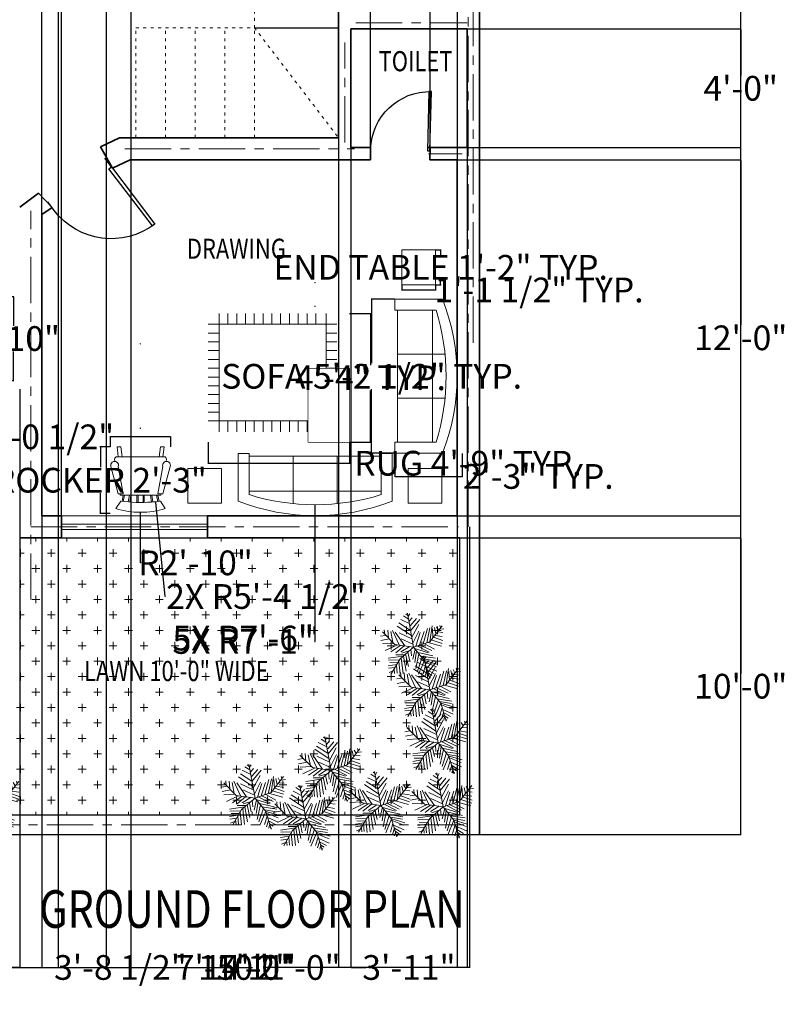
# Model space of a CAD drawing. Units: inches. Extents: x 541 to 1172, y -20 to 887.
# Tile 2 of 8: x 851 to 1162, y -20 to 378. Entities that reach past the tile are written whole.
import ezdxf

# ---------------------------------------------------------------- set-up
doc = ezdxf.new("R2010")
doc.units = ezdxf.units.IN
doc.header["$MEASUREMENT"] = 0
doc.set_wipeout_variables(frame=1)
doc.linetypes.add('ACAD_ISO03W100', pattern=[30, 12, -18])
doc.linetypes.add('CENTER', pattern=[50.8, 31.75, -6.35, 6.35, -6.35])
doc.layers.get('0').update_dxf_attribs({"color": 70})
for name, color, linetype, lineweight in [('A-ANNO-DIMS', 2, 'Continuous', 18), ('A-ANNO-TEXT', 7, 'Continuous', 30), ('A-AREA-IDEN', 7, 'Continuous', 20), ('A-DOOR', 4, 'Continuous', 25), ('A-FLOR-STRS-HIDN', 131, 'ACAD_ISO03W100', 18), ('A-FURN', 30, 'Continuous', 18), ('A-WALL-CNTR', 1, 'CENTER', 13), ('C-PROP', 7, 'Continuous', 25), ('L-PLNT', 70, 'Continuous', 18), ('L-PLNT-PATT', 70, 'Continuous', 13), ('L-SITE-WALL', 7, 'Continuous', 30), ('STAIRS', 131, 'Continuous', 25), ('WALL', 7, 'Continuous', 35), ('WINDOW', 2, 'Continuous', 18)]:
    doc.layers.add(name, color=color, linetype=linetype, lineweight=lineweight)
doc.styles.get("Standard").update_dxf_attribs({"font": 'arial.ttf'})
doc.styles.add('YQ_DIM', font='SUPEROS.SHX', dxfattribs={"width": 0.8, "bigfont": 'HZDX.SHX'})
doc.dimstyles.get("Standard").update_dxf_attribs({"dimtxt": 10, "dimasz": 0.18, "dimexe": 0.18, "dimexo": 0.0625, "dimgap": 0.09, "dimtad": 0, "dimtih": 1, "dimtoh": 1, "dimdec": 1, "dimzin": 0, "dimdsep": 46, "dimlunit": 4, "dimtxsty": 'Standard', "dimcen": 0.09, "dimadec": 0, "dimazin": 0, "dimtfac": 1, "dimtdec": 1, "dimtofl": 0, "dimtmove": 0, "dimatfit": 3, "dimfxl": 1, "dimtolj": 1, "dimtzin": 0, "dimarcsym": 0})

# ---------------------------------------------------------------- blocks, each defined once
blk = doc.blocks.new('*U7')
for p, q in [((-8.737, 47.138), (-17.069, 52.711)), ((-10.186, 53.64), (-13.084, 55.962)), ((0, 0), (-10.5, 57)), ((-9.099, 51.782), (-6.563, 55.962)), ((-3.665, 19.273), (-27.574, 35.527)), ((-5.114, 28.097), (-24.676, 40.636)), ((-7.288, 39.707), (-21.778, 46.673)), ((-7.65, 43.423), (-2.578, 49.46)), ((-5.839, 35.992), (4.667, 48.067)), ((-5.114, 27.632), (10.463, 46.673)), ((-2.941, 16.486), (8.652, 37.85)), ((27, 9), (48, 36)), ((27.127, 9.056), (31.112, 35.992)), ((38.719, 34.134), (41.979, 28.561)), ((44.153, 36.456), (45.239, 32.741)), ((-47.498, 19.737), (-55.83, 18.344)), ((-31.5, 4.5), (-52.5, 25.5)), ((-48.585, 21.131), (-49.309, 29.026)), ((-43.513, 28.561), (-42.427, 15.558)), ((-38.442, 26.239), (-34.819, 7.663)), ((-35.544, 28.097), (-24.314, 3.947)), ((-14.533, 2.09), (-30.834, 25.31)), ((-24.314, 23.917), (-2.941, 13.7)), ((-1.129, 6.734), (9.014, 26.704)), ((3.942, 1.625), (11.187, 24.381)), ((10.101, 3.483), (17.708, 26.239)), ((16.259, 5.805), (23.142, 31.348)), ((22.055, 7.198), (27.489, 32.277)), ((31.836, 30.883), (32.561, 16.486)), ((35.096, 32.741), (37.27, 22.524)), ((36.183, 19.737), (48.137, 17.88)), ((40.53, 25.775), (48.862, 24.846)), ((43.791, 29.954), (51.036, 30.883)), ((-40.615, 13.7), (-55.105, 10.913)), ((-33.37, 6.269), (-52.207, 5.34)), ((-28.299, 3.483), (-47.86, -5.805)), ((-21.416, 3.018), (-38.079, -8.128)), ((0, 0), (-31.5, 4.5)), ((-15.982, 2.09), (-30.11, -9.521)), ((0, 0), (-22.5, -19.5)), ((-6.563, 1.161), (-21.416, -8.128)), ((-20.691, 13.7), (-1.129, 4.876)), ((0, 0), (27, 9)), ((0, 0), (18, -22.5)), ((6.478, 1.625), (26.04, -8.592)), ((11.187, 3.483), (30.749, -5.805)), ((18.07, 5.805), (35.096, -3.483)), ((24.229, 7.663), (46.688, 1.625)), ((29.662, 12.307), (48.137, 6.269)), ((33.285, 16.486), (48.862, 10.913)), ((-17.431, -15.094), (-42.789, -18.809)), ((-15.257, -12.772), (-30.11, -12.772)), ((-6.563, -5.805), (-19.967, -9.985)), ((-17.069, -15.094), (-12.721, -40.172)), ((-13.446, -11.378), (-8.737, -32.741)), ((-9.461, -8.592), (-6.201, -23.453)), ((-4.752, -3.483), (-3.665, -14.629)), ((2.493, -3.019), (-1.491, -20.202)), ((1.769, -2.555), (24.229, -9.521)), ((5.029, -6.27), (2.131, -25.775)), ((9.014, -11.378), (3.58, -35.992)), ((7.565, -9.056), (32.198, -14.629)), ((12.274, -15.094), (36.907, -18.809)), ((-28.299, -29.026), (-42.789, -31.348)), ((-24.314, -21.596), (-42.427, -22.06)), ((-26.849, -26.24), (-40.253, -25.775)), ((-22.5, -19.5), (-37.5, -45)), ((-29.023, -30.884), (-27.936, -43.887)), ((-25.038, -23.918), (-22.865, -45.281)), ((-20.691, -18.345), (-17.793, -44.352)), ((14.085, -16.951), (6.478, -40.172)), ((18.07, -22.524), (8.289, -45.745)), ((20.244, -30.419), (15.897, -44.816)), ((16.259, -19.738), (36.183, -22.989)), ((18, -22.5), (27, -52.5)), ((18.433, -22.524), (40.53, -29.026)), ((19.157, -25.311), (38.719, -33.206)), ((21.331, -32.741), (39.081, -40.636)), ((-30.834, -34.135), (-42.427, -35.528)), ((-34.457, -39.708), (-40.978, -42.494)), ((-32.646, -36.921), (-31.921, -44.352)), ((22.78, -37.85), (19.519, -48.532)), ((22.78, -38.314), (34.372, -44.816)), ((24.591, -45.745), (23.142, -50.854)), ((24.591, -43.423), (30.749, -47.603)), ((26.764, -49.925), (28.213, -50.854))]:
    blk.add_line(p, q)
blk = doc.blocks.new('Sofa - Roundback 7 ft.')
for p, q in [((-12.00002, -32.4421), (-12.00003, -6.5971)), ((11.99997, -32.4421), (11.99998, -6.5971)), ((-36.000027, -34), (-36.000027, -11.4696)), ((-35.999844, -13.3819), (35.9998, -13.3819)), ((35.99998, -34), (35.99998, -11.4696)), ((-36.000027, -32.4421), (35.99998, -32.4421))]:
    blk.add_line(p, q)
for points in [[(-36.000027, -34), (-42.000027, -34), (-42.000027, -8)], [(41.99998, -8), (41.99998, -34), (35.99998, -34)]]:
    blk.add_lwpolyline(points)
for centre, radius, start, end in [((0, -114.25), 114.25, 68.43141, 111.5686), ((-0.00001, -127.1968), 121.1968, 72.72033, 107.2797)]:
    blk.add_arc(centre, radius, start, end)
blk = doc.blocks.new('Chair - Rocking')
for p, q in [((-8, -4.5), (-10, -1.5)), ((8, -4.5), (10, -1.5)), ((-9, -7.5), (-12, -18.49999)), ((-7, -7.5), (-9, -7.5)), ((-9, -18.49999), (-7, -7.5)), ((-8.23428, -6.99939), (-8.3093, -7.47958)), ((-8.23041, -7), (8.23915, -7)), ((-7.5, -4.5), (-7, -7)), ((-6.5, -7), (-7.02225, -4.43)), ((-4.5, -7), (-4.96674, -4.19951)), ((-4, -7), (-4.40532, -4.16272)), ((-1.5, -4.05012), (-1.5, -7)), ((-1, -7), (-1, -4.05012)), ((1, -7), (1, -4.04655)), ((1.5, -4.05012), (1.5, -7)), ((4, -7), (4.40187, -4.18694)), ((4.5, -7), (4.96761, -4.19437)), ((6.5, -7), (7, -4.4057)), ((7.5, -4.5), (7, -7)), ((7, -7.5), (9, -7.5)), ((9, -18.49999), (7, -7.5)), ((8.31071, -7.48854), (8.23449, -7.00073)), ((9, -7.5), (12, -18.49999)), ((-10.36644, -20.64523), (-10.5, -21.49999)), ((-9, -22.49999), (-9.5, -26.49999)), ((0, -22.49999), (-9.5, -22.49999)), ((-8, -26.49999), (-7.5, -22.49999)), ((0, -22.49999), (9.5, -22.49999)), ((8, -26.49999), (7.5, -22.49999)), ((9, -22.49999), (9.5, -26.49999)), ((10.5, -21.49999), (10.3575, -20.58798)), ((-9.5, -26.49999), (-8, -26.49999)), ((9.5, -26.49999), (8, -26.49999))]:
    blk.add_line(p, q)
for centre, radius, start, end in [((0, -34.08333), 34.08333, 72.93847, 107.0615), ((0, -68.25004), 64.25, 93.92211, 97.15267), ((0, -68.25004), 64.25, 82.84733, 93.92211), ((-10.5, -18.99999), 1.58114, 161.5651, 18.43495), ((10.5, -18.99999), 1.58114, 161.5651, 18.43495), ((-9.5, -21.49999), 1, 180, 270), ((9.5, -21.49999), 1, 270, 0)]:
    blk.add_arc(centre, radius, start, end)
blk = doc.blocks.new('*U23')
for p, q in [((0, 0), (0, -6)), ((40, 0), (40, -6))]:
    blk.add_line(p, q)
blk.add_lwpolyline([(0, 0), (0, 40), (1.75, 40), (1.75, 0)], close=True)
blk.add_arc((0, 0), 40, 0, 90)
blk = doc.blocks.new('*U26')
for p, q in [((0, 0), (0, 6)), ((40, 0), (40, 6))]:
    blk.add_line(p, q)
blk.add_lwpolyline([(0, 0), (0, -40), (1.75, -40), (1.75, 0)], close=True)
blk.add_arc((0, 0), 40, 270, 0)
blk = doc.blocks.new('WD_WIN4')
at = {"lineweight": -2}
for p, q in [((-0.5, 0.5), (0.5, 0.5)), ((-0.5, 0.12), (0.5, 0.12)), ((-0.5, -0.12), (0.5, -0.12)), ((-0.5, -0.5), (0.5, -0.5))]:
    blk.add_line(p, q, dxfattribs=at)
blk = doc.blocks.new('RUG-FRINGED-WITH-LOW-TABLE')
for p, q in [((4.37, 52.04), (4.37, 47.68)), ((7.93, 52.04), (7.93, 47.68)), ((11.48, 52.04), (11.48, 47.68)), ((15.04, 52.04), (15.04, 47.68)), ((18.6, 52.04), (18.6, 47.68)), ((22.16, 52.04), (22.16, 47.68)), ((25.72, 52.04), (25.72, 47.68)), ((29.27, 52.04), (29.27, 47.68)), ((32.83, 52.04), (32.83, 47.68)), ((36.39, 52.04), (36.39, 47.68)), ((39.95, 52.04), (39.95, 47.68)), ((43.51, 52.04), (43.51, 47.68)), ((47.65, 52.04), (47.65, 47.68)), ((4.37, 47.68), (0, 47.68)), ((4.37, 44.12), (0, 44.12)), ((47.65, 47.68), (52.02, 47.68)), ((47.65, 44.12), (52.02, 44.12)), ((4.37, 40.56), (0, 40.56)), ((47.65, 40.56), (52.02, 40.56)), ((4.37, 37), (0, 37)), ((47.65, 37), (52.02, 37)), ((4.37, 33.44), (0, 33.44)), ((47.65, 33.44), (52.02, 33.44)), ((4.37, 29.89), (0, 29.89)), ((47.65, 29.89), (52.02, 29.89)), ((4.37, 26.33), (0, 26.33)), ((47.65, 26.33), (52.02, 26.33)), ((4.37, 22.77), (0, 22.77)), ((47.65, 22.77), (52.02, 22.77)), ((4.37, 19.21), (0, 19.21)), ((47.65, 19.21), (52.02, 19.21)), ((4.37, 15.65), (0, 15.65)), ((4.37, 12.1), (0, 12.1)), ((47.65, 15.65), (52.02, 15.65)), ((47.65, 12.1), (52.02, 12.1)), ((4.37, 8.54), (0, 8.54)), ((4.37, 4.17), (4.37, 8.54)), ((7.93, 4.17), (7.93, 8.54)), ((11.48, 4.17), (11.48, 8.54)), ((15.04, 4.17), (15.04, 8.54)), ((18.6, 4.17), (18.6, 8.54)), ((22.16, 4.17), (22.16, 8.54)), ((25.72, 4.17), (25.72, 8.54)), ((29.27, 4.17), (29.27, 8.54)), ((32.83, 4.17), (32.83, 8.54)), ((36.39, 4.17), (36.39, 8.54)), ((39.95, 4.17), (39.95, 8.54)), ((43.51, 4.17), (43.51, 8.54)), ((47.65, 8.54), (52.02, 8.54)), ((47.65, 4.17), (47.65, 8.54))]:
    blk.add_line(p, q)
for points in [[(4.37, 47.68), (47.65, 47.68), (47.65, 8.54), (4.37, 8.54)], [(40.42, 29.74), (57.09, 29.74), (57.09, 0), (40.42, 0)]]:
    blk.add_lwpolyline(points, close=True)
blk.add_wipeout([(57.09, 0), (40.42, 0), (40.42, 29.74), (57.09, 29.74), (57.09, 29.74)])
blk = doc.blocks.new('FURN-END-TABLE')
blk.add_lwpolyline([(0, 14.11), (13.62, 14.11), (13.62, 0), (0, 0)], close=True)
blk = doc.blocks.new('*D37')
at = {"layer": 'A-ANNO-DIMS', "color": 0, "lineweight": -2, "transparency": 16777216}
for p, q in [((1002.98, 265.26), (993.51, 265.26)), ((993.69, 265.08), (993.69, 239.34)), ((993.69, 203.08), (993.69, 228.81)), ((1002.98, 202.9), (993.51, 202.9))]:
    blk.add_line(p, q, dxfattribs=at)
for points in [[(993.66, 265.08), (993.72, 265.08), (993.69, 265.26)], [(993.66, 203.08), (993.72, 203.08), (993.69, 202.9)]]:
    blk.add_solid(points, dxfattribs=at)
at = {"layer": 'Defpoints', "color": 0, "lineweight": -2, "transparency": 16777216}
for p in [(1003.04, 265.26), (993.69, 202.9), (1003.04, 202.9)]:
    blk.add_point(p, dxfattribs=at)
at = {"layer": 'A-ANNO-DIMS', "color": 0, "transparency": 16777216, "insert": (993.69, 234.08), "char_height": 10, "attachment_point": 5}
blk.add_mtext('\\A1;SOFA 5\'-2 1/2" TYP.', dxfattribs=at)
blk = doc.blocks.new('*D38')
at = {"layer": 'A-ANNO-DIMS', "color": 0, "lineweight": -2, "transparency": 16777216}
for p, q in [((1003.04, 202.83), (1003.04, 193.36)), ((1030.26, 202.83), (1030.26, 193.36)), ((1003.22, 193.54), (1030.08, 193.54)), ((1030.26, 193.54), (1030.44, 193.54))]:
    blk.add_line(p, q, dxfattribs=at)
for points in [[(1003.22, 193.57), (1003.22, 193.51), (1003.04, 193.54)], [(1030.08, 193.57), (1030.08, 193.51), (1030.26, 193.54)]]:
    blk.add_solid(points, dxfattribs=at)
at = {"layer": 'Defpoints', "color": 0, "lineweight": -2, "transparency": 16777216}
for p in [(1003.04, 202.9), (1030.26, 202.9), (1030.26, 193.54)]:
    blk.add_point(p, dxfattribs=at)
at = {"layer": 'A-ANNO-DIMS', "color": 0, "transparency": 16777216, "insert": (1061.1, 193.54), "char_height": 10, "attachment_point": 5}
blk.add_mtext('\\A1;2\'-3" TYP.', dxfattribs=at)
blk = doc.blocks.new('*D47')
at = {"layer": 'A-ANNO-DIMS', "color": 0, "lineweight": -2, "transparency": 16777216}
for p, q in [((1019.56, 285.25), (1021.8, 285.25)), ((1021.62, 285.07), (1021.62, 283.3)), ((1019.56, 271.13), (1021.8, 271.13)), ((1021.62, 271.31), (1021.62, 273.08))]:
    blk.add_line(p, q, dxfattribs=at)
for points in [[(1021.59, 285.07), (1021.65, 285.07), (1021.62, 285.25)], [(1021.59, 271.31), (1021.65, 271.31), (1021.62, 271.13)]]:
    blk.add_solid(points, dxfattribs=at)
at = {"layer": 'Defpoints', "color": 0, "lineweight": -2, "transparency": 16777216}
for p in [(1019.5, 285.25), (1021.62, 285.25), (1019.5, 271.13)]:
    blk.add_point(p, dxfattribs=at)
at = {"layer": 'A-ANNO-DIMS', "color": 0, "transparency": 16777216, "insert": (1021.62, 278.19), "char_height": 10, "attachment_point": 5}
blk.add_mtext('\\A1;END TABLE 1\'-2" TYP.', dxfattribs=at)
blk = doc.blocks.new('*D48')
at = {"layer": 'A-ANNO-DIMS', "color": 0, "lineweight": -2, "transparency": 16777216}
for p, q in [((1005.88, 271.07), (1005.88, 268.84)), ((1019.5, 271.07), (1019.5, 268.84)), ((1006.06, 269.02), (1019.32, 269.02)), ((1019.5, 269.02), (1019.68, 269.02))]:
    blk.add_line(p, q, dxfattribs=at)
for points in [[(1006.06, 269.05), (1006.06, 268.99), (1005.88, 269.02)], [(1019.32, 269.05), (1019.32, 268.99), (1019.5, 269.02)]]:
    blk.add_solid(points, dxfattribs=at)
at = {"layer": 'Defpoints', "color": 0, "lineweight": -2, "transparency": 16777216}
for p in [(1005.88, 271.13), (1019.5, 271.13), (1019.5, 269.02)]:
    blk.add_point(p, dxfattribs=at)
at = {"layer": 'A-ANNO-DIMS', "color": 0, "transparency": 16777216, "insert": (1061.43, 269.02), "char_height": 10, "attachment_point": 5}
blk.add_mtext('\\A1;1\'-1 1/2" TYP.', dxfattribs=at)
blk = doc.blocks.new('*D59')
at = {"layer": 'A-ANNO-DIMS', "color": 0, "lineweight": -2, "transparency": 16777216}
for p, q in [((927.6, 207.39), (927.6, 198.71)), ((984.69, 207.39), (984.69, 198.71)), ((927.78, 198.89), (984.51, 198.89)), ((984.69, 198.89), (984.87, 198.89))]:
    blk.add_line(p, q, dxfattribs=at)
for points in [[(927.78, 198.92), (927.78, 198.86), (927.6, 198.89)], [(984.51, 198.92), (984.51, 198.86), (984.69, 198.89)]]:
    blk.add_solid(points, dxfattribs=at)
at = {"layer": 'Defpoints', "color": 0, "lineweight": -2, "transparency": 16777216}
for p in [(927.6, 207.45), (984.69, 207.45), (984.69, 198.89)]:
    blk.add_point(p, dxfattribs=at)
at = {"layer": 'A-ANNO-DIMS', "color": 0, "transparency": 16777216, "insert": (1032.64, 198.89), "char_height": 10, "attachment_point": 5}
blk.add_mtext('\\A1;RUG 4\'-9" TYP.', dxfattribs=at)
blk = doc.blocks.new('*D60')
at = {"layer": 'A-ANNO-DIMS', "color": 0, "lineweight": -2, "transparency": 16777216}
for p, q in [((984.75, 259.5), (993.43, 259.5)), ((993.25, 259.32), (993.25, 238.57)), ((993.25, 207.63), (993.25, 228.38)), ((984.75, 207.45), (993.43, 207.45))]:
    blk.add_line(p, q, dxfattribs=at)
for points in [[(993.22, 259.32), (993.28, 259.32), (993.25, 259.5)], [(993.22, 207.63), (993.28, 207.63), (993.25, 207.45)]]:
    blk.add_solid(points, dxfattribs=at)
at = {"layer": 'Defpoints', "color": 0, "lineweight": -2, "transparency": 16777216}
for p in [(984.69, 259.5), (993.25, 259.5), (984.69, 207.45)]:
    blk.add_point(p, dxfattribs=at)
at = {"layer": 'A-ANNO-DIMS', "color": 0, "transparency": 16777216, "insert": (993.25, 233.47), "char_height": 10, "attachment_point": 5}
blk.add_mtext('\\A1;4\'-4" TYP.', dxfattribs=at)
blk = doc.blocks.new('*D63')
at = {"layer": 'A-ANNO-DIMS', "color": 0, "lineweight": -2, "transparency": 16777216}
for p, q in [((887.91, 205.52), (883.75, 205.52)), ((883.93, 205.34), (883.93, 197.29)), ((883.93, 178.7), (883.93, 186.75)), ((887.91, 178.52), (883.75, 178.52))]:
    blk.add_line(p, q, dxfattribs=at)
for points in [[(883.9, 205.34), (883.96, 205.34), (883.93, 205.52)], [(883.9, 178.7), (883.96, 178.7), (883.93, 178.52)]]:
    blk.add_solid(points, dxfattribs=at)
at = {"layer": 'Defpoints', "color": 0, "lineweight": -2, "transparency": 16777216}
for p in [(887.98, 205.52), (883.93, 178.52), (887.98, 178.52)]:
    blk.add_point(p, dxfattribs=at)
at = {"layer": 'A-ANNO-DIMS', "color": 0, "transparency": 16777216, "insert": (883.93, 192.02), "char_height": 10, "attachment_point": 5}
blk.add_mtext('\\A1;ROCKER 2\'-3"', dxfattribs=at)
blk = doc.blocks.new('*D64')
at = {"layer": 'A-ANNO-DIMS', "color": 0, "lineweight": -2, "transparency": 16777216}
for p, q in [((887.98, 209.57), (887.8, 209.57)), ((887.98, 205.58), (887.98, 209.75)), ((912.23, 209.57), (888.16, 209.57)), ((912.41, 205.58), (912.41, 209.75))]:
    blk.add_line(p, q, dxfattribs=at)
for points in [[(888.16, 209.6), (888.16, 209.54), (887.98, 209.57)], [(912.23, 209.6), (912.23, 209.54), (912.41, 209.57)]]:
    blk.add_solid(points, dxfattribs=at)
at = {"layer": 'Defpoints', "color": 0, "lineweight": -2, "transparency": 16777216}
for p in [(887.98, 209.57), (887.98, 205.52), (912.41, 205.52)]:
    blk.add_point(p, dxfattribs=at)
at = {"layer": 'A-ANNO-DIMS', "color": 0, "transparency": 16777216, "insert": (862.68, 209.57), "char_height": 10, "attachment_point": 5}
blk.add_mtext('\\A1;2\'-0 1/2"', dxfattribs=at)
blk = doc.blocks.new('*D68')
at = {"layer": 'A-ANNO-DIMS', "color": 0, "lineweight": -2, "transparency": 16777216}
for p, q in [((843.47, 266.37), (848.9, 266.37)), ((848.72, 266.19), (848.72, 254.56)), ((848.72, 232.53), (848.72, 244.17)), ((843.47, 232.35), (848.9, 232.35))]:
    blk.add_line(p, q, dxfattribs=at)
for points in [[(848.69, 266.19), (848.75, 266.19), (848.72, 266.37)], [(848.69, 232.53), (848.75, 232.53), (848.72, 232.35)]]:
    blk.add_solid(points, dxfattribs=at)
at = {"layer": 'Defpoints', "color": 0, "lineweight": -2, "transparency": 16777216}
for p in [(843.41, 266.37), (848.72, 266.37), (843.41, 232.35)]:
    blk.add_point(p, dxfattribs=at)
at = {"layer": 'A-ANNO-DIMS', "color": 0, "transparency": 16777216, "insert": (848.72, 249.36), "char_height": 10, "attachment_point": 5}
blk.add_mtext('\\A1;2\'-10"', dxfattribs=at)
blk = doc.blocks.new('*D70')
at = {"layer": 'A-ANNO-DIMS', "color": 0, "lineweight": -2, "transparency": 16777216}
for p, q in [((1036.7, 829.68), (1143.21, 829.68)), ((1143.03, 829.5), (1143.03, 444.36)), ((1143.03, 48.83), (1143.03, 433.97)), ((1037.35, 48.65), (1143.21, 48.65))]:
    blk.add_line(p, q, dxfattribs=at)
for points in [[(1143, 829.5), (1143.06, 829.5), (1143.03, 829.68)], [(1143, 48.83), (1143.06, 48.83), (1143.03, 48.65)]]:
    blk.add_solid(points, dxfattribs=at)
at = {"layer": 'Defpoints', "color": 0, "lineweight": -2, "transparency": 16777216}
for p in [(1036.64, 829.68), (1037.28, 48.65), (1143.03, 48.65)]:
    blk.add_point(p, dxfattribs=at)
at = {"layer": 'A-ANNO-DIMS', "color": 0, "transparency": 16777216, "insert": (1143.03, 439.17), "char_height": 10, "attachment_point": 5}
blk.add_mtext('\\A1;65\'-1"', dxfattribs=at)
blk = doc.blocks.new('*D72')
at = {"layer": 'A-ANNO-DIMS', "color": 0, "lineweight": -2, "transparency": 16777216}
for p, q in [((676.28, 228.86), (676.28, -5.37)), ((851.28, 228.86), (851.28, -5.37)), ((676.46, -5.19), (746.99, -5.19)), ((851.1, -5.19), (780.58, -5.19))]:
    blk.add_line(p, q, dxfattribs=at)
for points in [[(676.46, -5.16), (676.46, -5.22), (676.28, -5.19)], [(851.1, -5.16), (851.1, -5.22), (851.28, -5.19)]]:
    blk.add_solid(points, dxfattribs=at)
at = {"layer": 'Defpoints', "color": 0, "lineweight": -2, "transparency": 16777216}
for p in [(676.28, 228.92), (851.28, 228.92), (851.28, -5.19)]:
    blk.add_point(p, dxfattribs=at)
at = {"layer": 'A-ANNO-DIMS', "color": 0, "transparency": 16777216, "insert": (763.78, -5.19), "char_height": 10, "attachment_point": 5}
blk.add_mtext('\\A1;14\'-7"', dxfattribs=at)
blk = doc.blocks.new('*D73')
at = {"layer": 'A-ANNO-DIMS', "color": 0, "lineweight": -2, "transparency": 16777216}
for p, q in [((1033.35, 173.09), (1033.35, -5.37)), ((851.28, 168.59), (851.28, -5.37)), ((851.46, -5.19), (925.52, -5.19)), ((1033.17, -5.19), (959.11, -5.19))]:
    blk.add_line(p, q, dxfattribs=at)
for points in [[(851.46, -5.16), (851.46, -5.22), (851.28, -5.19)], [(1033.17, -5.16), (1033.17, -5.22), (1033.35, -5.19)]]:
    blk.add_solid(points, dxfattribs=at)
at = {"layer": 'Defpoints', "color": 0, "lineweight": -2, "transparency": 16777216}
for p in [(1033.35, 173.15), (851.28, 168.65), (1033.35, -5.19)]:
    blk.add_point(p, dxfattribs=at)
at = {"layer": 'A-ANNO-DIMS', "color": 0, "transparency": 16777216, "insert": (942.31, -5.19), "char_height": 10, "attachment_point": 5}
blk.add_mtext('\\A1;15\'-2"', dxfattribs=at)
blk = doc.blocks.new('*D86')
at = {"layer": 'A-ANNO-DIMS', "color": 0, "lineweight": -2, "transparency": 16777216}
for p, q in [((896.28, 439.59), (896.28, -5.37)), ((1028.28, 439.59), (1028.28, -5.37)), ((896.46, -5.19), (945.49, -5.19)), ((1028.1, -5.19), (979.08, -5.19))]:
    blk.add_line(p, q, dxfattribs=at)
for points in [[(896.46, -5.16), (896.46, -5.22), (896.28, -5.19)], [(1028.1, -5.16), (1028.1, -5.22), (1028.28, -5.19)]]:
    blk.add_solid(points, dxfattribs=at)
at = {"layer": 'Defpoints', "color": 0, "lineweight": -2, "transparency": 16777216}
for p in [(896.28, 439.65), (1028.28, 439.65), (1028.28, -5.19)]:
    blk.add_point(p, dxfattribs=at)
at = {"layer": 'A-ANNO-DIMS', "color": 0, "transparency": 16777216, "insert": (962.28, -5.19), "char_height": 10, "attachment_point": 5}
blk.add_mtext('\\A1;11\'-0"', dxfattribs=at)
blk = doc.blocks.new('*D90')
at = {"layer": 'A-ANNO-DIMS', "color": 0, "lineweight": -2, "transparency": 16777216}
for p, q in [((1032.35, 374.65), (1143.21, 374.65)), ((1143.03, 374.47), (1143.03, 355.85)), ((1143.03, 326.83), (1143.03, 345.46)), ((1032.35, 326.65), (1143.21, 326.65))]:
    blk.add_line(p, q, dxfattribs=at)
for points in [[(1143, 374.47), (1143.06, 374.47), (1143.03, 374.65)], [(1143, 326.83), (1143.06, 326.83), (1143.03, 326.65)]]:
    blk.add_solid(points, dxfattribs=at)
at = {"layer": 'Defpoints', "color": 0, "lineweight": -2, "transparency": 16777216}
for p in [(1032.28, 374.65), (1032.28, 326.65), (1143.03, 326.65)]:
    blk.add_point(p, dxfattribs=at)
at = {"layer": 'A-ANNO-DIMS', "color": 0, "transparency": 16777216, "insert": (1143.03, 350.65), "char_height": 10, "attachment_point": 5}
blk.add_mtext('\\A1;4\'-0"', dxfattribs=at)
blk = doc.blocks.new('*D91')
at = {"layer": 'A-ANNO-DIMS', "color": 0, "lineweight": -2, "transparency": 16777216}
for p, q in [((985.28, 374.59), (985.28, -5.37)), ((1032.28, 374.59), (1032.28, -5.37)), ((985.46, -5.19), (991.52, -5.19)), ((1032.1, -5.19), (1026.05, -5.19))]:
    blk.add_line(p, q, dxfattribs=at)
for points in [[(985.46, -5.16), (985.46, -5.22), (985.28, -5.19)], [(1032.1, -5.16), (1032.1, -5.22), (1032.28, -5.19)]]:
    blk.add_solid(points, dxfattribs=at)
at = {"layer": 'Defpoints', "color": 0, "lineweight": -2, "transparency": 16777216}
for p in [(985.28, 374.65), (1032.28, 374.65), (1032.28, -5.19)]:
    blk.add_point(p, dxfattribs=at)
at = {"layer": 'A-ANNO-DIMS', "color": 0, "transparency": 16777216, "insert": (1008.78, -5.19), "char_height": 10, "attachment_point": 5}
blk.add_mtext('\\A1;3\'-11"', dxfattribs=at)
blk = doc.blocks.new('*D93')
at = {"layer": 'A-ANNO-DIMS', "color": 0, "lineweight": -2, "transparency": 16777216}
for p, q in [((860.28, 177.59), (860.28, -5.37)), ((1028.28, 177.59), (1028.28, -5.37)), ((860.46, -5.19), (927.49, -5.19)), ((1028.1, -5.19), (961.08, -5.19))]:
    blk.add_line(p, q, dxfattribs=at)
for points in [[(860.46, -5.16), (860.46, -5.22), (860.28, -5.19)], [(1028.1, -5.16), (1028.1, -5.22), (1028.28, -5.19)]]:
    blk.add_solid(points, dxfattribs=at)
at = {"layer": 'Defpoints', "color": 0, "lineweight": -2, "transparency": 16777216}
for p in [(860.28, 177.65), (1028.28, 177.65), (1028.28, -5.19)]:
    blk.add_point(p, dxfattribs=at)
at = {"layer": 'A-ANNO-DIMS', "color": 0, "transparency": 16777216, "insert": (944.28, -5.19), "char_height": 10, "attachment_point": 5}
blk.add_mtext('\\A1;14\'-0"', dxfattribs=at)
blk = doc.blocks.new('*D94')
at = {"layer": 'A-ANNO-DIMS', "color": 0, "lineweight": -2, "transparency": 16777216}
for p, q in [((1028.35, 321.65), (1143.21, 321.65)), ((1143.03, 321.47), (1143.03, 254.85)), ((1143.03, 177.83), (1143.03, 244.46)), ((1028.35, 177.65), (1143.21, 177.65))]:
    blk.add_line(p, q, dxfattribs=at)
for points in [[(1143, 321.47), (1143.06, 321.47), (1143.03, 321.65)], [(1143, 177.83), (1143.06, 177.83), (1143.03, 177.65)]]:
    blk.add_solid(points, dxfattribs=at)
at = {"layer": 'Defpoints', "color": 0, "lineweight": -2, "transparency": 16777216}
for p in [(1028.28, 321.65), (1143.03, 321.65), (1028.28, 177.65)]:
    blk.add_point(p, dxfattribs=at)
at = {"layer": 'A-ANNO-DIMS', "color": 0, "transparency": 16777216, "insert": (1143.03, 249.65), "char_height": 10, "attachment_point": 5}
blk.add_mtext('\\A1;12\'-0"', dxfattribs=at)
blk = doc.blocks.new('*D95')
at = {"layer": 'A-ANNO-DIMS', "color": 0, "lineweight": -2, "transparency": 16777216}
for p, q in [((886.28, 385.11), (886.28, -5.37)), ((980.28, 385.11), (980.28, -5.37)), ((886.46, -5.19), (916.06, -5.19)), ((980.1, -5.19), (950.51, -5.19))]:
    blk.add_line(p, q, dxfattribs=at)
for points in [[(886.46, -5.16), (886.46, -5.22), (886.28, -5.19)], [(980.1, -5.16), (980.1, -5.22), (980.28, -5.19)]]:
    blk.add_solid(points, dxfattribs=at)
at = {"layer": 'Defpoints', "color": 0, "lineweight": -2, "transparency": 16777216}
for p in [(886.28, 385.17), (980.28, 385.17), (980.28, -5.19)]:
    blk.add_point(p, dxfattribs=at)
at = {"layer": 'A-ANNO-DIMS', "color": 0, "transparency": 16777216, "insert": (933.28, -5.19), "char_height": 10, "attachment_point": 5}
blk.add_mtext('\\A1;7\'-10"', dxfattribs=at)
blk = doc.blocks.new('*D98')
at = {"layer": 'A-ANNO-DIMS', "color": 0, "lineweight": -2, "transparency": 16777216}
for p, q in [((993.28, 326.72), (993.28, 872.66)), ((993.46, 872.48), (1017.14, 872.48)), ((1017.32, 326.72), (1017.32, 872.66)), ((1017.32, 872.48), (1017.5, 872.48))]:
    blk.add_line(p, q, dxfattribs=at)
for points in [[(993.46, 872.51), (993.46, 872.45), (993.28, 872.48)], [(1017.14, 872.51), (1017.14, 872.45), (1017.32, 872.48)]]:
    blk.add_solid(points, dxfattribs=at)
at = {"layer": 'Defpoints', "color": 0, "lineweight": -2, "transparency": 16777216}
for p in [(1017.32, 872.48), (993.28, 326.65), (1017.32, 326.65)]:
    blk.add_point(p, dxfattribs=at)
at = {"layer": 'A-ANNO-DIMS', "color": 0, "transparency": 16777216, "insert": (1030.97, 872.48), "char_height": 10, "attachment_point": 5}
blk.add_mtext('\\A1;2\'-0"', dxfattribs=at)
blk = doc.blocks.new('*D102')
at = {"layer": 'A-ANNO-DIMS', "color": 0, "lineweight": -2, "transparency": 16777216}
for p, q in [((822.26, 582.59), (822.26, -5.37)), ((866.83, 582.59), (866.83, -5.37)), ((822.44, -5.19), (866.65, -5.19)), ((866.83, -5.19), (867.01, -5.19))]:
    blk.add_line(p, q, dxfattribs=at)
for points in [[(822.44, -5.16), (822.44, -5.22), (822.26, -5.19)], [(866.65, -5.16), (866.65, -5.22), (866.83, -5.19)]]:
    blk.add_solid(points, dxfattribs=at)
at = {"layer": 'Defpoints', "color": 0, "lineweight": -2, "transparency": 16777216}
for p in [(822.26, 582.65), (866.83, 582.65), (866.83, -5.19)]:
    blk.add_point(p, dxfattribs=at)
at = {"layer": 'A-ANNO-DIMS', "color": 0, "transparency": 16777216, "insert": (892.04, -5.19), "char_height": 10, "attachment_point": 5}
blk.add_mtext('\\A1;3\'-8 1/2"', dxfattribs=at)
blk = doc.blocks.new('*D104')
at = {"layer": 'A-ANNO-DIMS', "color": 0, "lineweight": -2, "transparency": 16777216}
for p, q in [((860.28, 177.72), (860.28, 872.66)), ((860.46, 872.48), (867.98, 872.48)), ((868.16, 177.72), (868.16, 872.66)), ((868.16, 872.48), (868.34, 872.48))]:
    blk.add_line(p, q, dxfattribs=at)
for points in [[(860.46, 872.51), (860.46, 872.45), (860.28, 872.48)], [(867.98, 872.51), (867.98, 872.45), (868.16, 872.48)]]:
    blk.add_solid(points, dxfattribs=at)
at = {"layer": 'Defpoints', "color": 0, "lineweight": -2, "transparency": 16777216}
for p in [(868.16, 872.48), (860.28, 177.65), (868.16, 177.65)]:
    blk.add_point(p, dxfattribs=at)
at = {"layer": 'A-ANNO-DIMS', "color": 0, "transparency": 16777216, "insert": (881.72, 872.48), "char_height": 10, "attachment_point": 5}
blk.add_mtext('\\A1;0\'-8"', dxfattribs=at)
blk = doc.blocks.new('*D109')
at = {"layer": 'A-ANNO-DIMS', "color": 0, "lineweight": -2, "transparency": 16777216}
for p, q in [((851.35, 168.65), (1143.21, 168.65)), ((1143.03, 168.47), (1143.03, 113.85)), ((1143.03, 48.83), (1143.03, 103.46)), ((1037.35, 48.65), (1143.21, 48.65))]:
    blk.add_line(p, q, dxfattribs=at)
for points in [[(1143, 168.47), (1143.06, 168.47), (1143.03, 168.65)], [(1143, 48.83), (1143.06, 48.83), (1143.03, 48.65)]]:
    blk.add_solid(points, dxfattribs=at)
at = {"layer": 'Defpoints', "color": 0, "lineweight": -2, "transparency": 16777216}
for p in [(851.28, 168.65), (1037.28, 48.65), (1143.03, 48.65)]:
    blk.add_point(p, dxfattribs=at)
at = {"layer": 'A-ANNO-DIMS', "color": 0, "transparency": 16777216, "insert": (1143.03, 108.65), "char_height": 10, "attachment_point": 5}
blk.add_mtext('\\A1;10\'-0"', dxfattribs=at)
blk = doc.blocks.new('*D111')
at = {"layer": 'A-ANNO-DIMS', "color": 0, "lineweight": -2, "transparency": 16777216}
for p, q in [((970.72, 272.09), (970.9, 272.09)), ((970.81, 272), (970.81, 272.18)), ((970.81, 128.12), (970.81, 181.93)), ((970.63, 128.12), (970.81, 128.12))]:
    blk.add_line(p, q, dxfattribs=at)
blk.add_solid([(970.78, 181.93), (970.84, 181.93), (970.81, 182.11)], dxfattribs=at)
at = {"layer": 'Defpoints', "color": 0, "lineweight": -2, "transparency": 16777216}
for p in [(970.81, 272.09), (970.81, 182.11)]:
    blk.add_point(p, dxfattribs=at)
at = {"layer": 'A-ANNO-DIMS', "color": 0, "transparency": 16777216, "insert": (941.72, 128.12), "char_height": 10, "attachment_point": 5}
blk.add_mtext('\\A1;5X R7\'-6"', dxfattribs=at)
blk = doc.blocks.new('*D112')
at = {"layer": 'A-ANNO-DIMS', "color": 0, "lineweight": -2, "transparency": 16777216}
for p, q in [((970.72, 262.48), (970.9, 262.48)), ((970.81, 262.39), (970.81, 262.57)), ((970.81, 126.76), (970.81, 177.47)), ((970.63, 126.76), (970.81, 126.76))]:
    blk.add_line(p, q, dxfattribs=at)
blk.add_solid([(970.78, 177.47), (970.84, 177.47), (970.81, 177.65)], dxfattribs=at)
at = {"layer": 'Defpoints', "color": 0, "lineweight": -2, "transparency": 16777216}
for p in [(970.81, 262.48), (970.81, 177.65)]:
    blk.add_point(p, dxfattribs=at)
at = {"layer": 'A-ANNO-DIMS', "color": 0, "transparency": 16777216, "insert": (941.72, 126.76), "char_height": 10, "attachment_point": 5}
blk.add_mtext('\\A1;5X R7\'-1"', dxfattribs=at)
blk = doc.blocks.new('*D113')
at = {"layer": 'A-ANNO-DIMS', "color": 0, "lineweight": -2, "transparency": 16777216}
for p, q in [((900.1, 247.27), (900.28, 247.27)), ((900.19, 247.18), (900.19, 247.36)), ((910.11, 144.95), (906.41, 183.14)), ((910.29, 144.95), (910.11, 144.95))]:
    blk.add_line(p, q, dxfattribs=at)
blk.add_solid([(906.44, 183.14), (906.38, 183.14), (906.39, 183.32)], dxfattribs=at)
at = {"layer": 'Defpoints', "color": 0, "lineweight": -2, "transparency": 16777216}
for p in [(900.19, 247.27), (906.39, 183.32)]:
    blk.add_point(p, dxfattribs=at)
at = {"layer": 'A-ANNO-DIMS', "color": 0, "transparency": 16777216, "insert": (950.94, 144.95), "char_height": 10, "attachment_point": 5}
blk.add_mtext('\\A1;2X R5\'-4 1/2"', dxfattribs=at)
blk = doc.blocks.new('*D114')
at = {"layer": 'A-ANNO-DIMS', "color": 0, "lineweight": -2, "transparency": 16777216}
for p, q in [((900.1, 213.1), (900.28, 213.1)), ((900.19, 213.01), (900.19, 213.19)), ((900.2, 158.57), (900.19, 178.84)), ((900.38, 158.57), (900.2, 158.57))]:
    blk.add_line(p, q, dxfattribs=at)
blk.add_solid([(900.23, 178.84), (900.17, 178.84), (900.19, 179.02)], dxfattribs=at)
at = {"layer": 'Defpoints', "color": 0, "lineweight": -2, "transparency": 16777216}
for p in [(900.19, 213.1), (900.19, 179.02)]:
    blk.add_point(p, dxfattribs=at)
at = {"layer": 'A-ANNO-DIMS', "color": 0, "transparency": 16777216, "insert": (922.43, 158.57), "char_height": 10, "attachment_point": 5}
blk.add_mtext('\\A1;R2\'-10"', dxfattribs=at)

msp = doc.modelspace()

# ---------------------------------------------------------------- hatches: boundary and pattern name
at = {"layer": 'L-PLNT-PATT'}
h = msp.add_hatch(dxfattribs=at)
h.set_pattern_fill('CROSS', color=256, scale=25)
h.paths.add_polyline_path([(851.28, 56.54), (821.61, 56.53), (821.61, 109.68), (851.28, 109.68), (851.28, 168.65), (1029.41, 168.65), (1029.41, 56.54)])
h.paths.add_polyline_path([(1021.4, 66.61), (1021.48, 66.56), (1021.42, 66.49)], flags=16)

# ---------------------------------------------------------------- linework, layer by layer
at = {"layer": 'A-FLOR-STRS-HIDN', "ltscale": 0.1}
for p, q in [((910.28, 330.65), (910.28, 375.17)), ((922.28, 330.65), (922.28, 375.17)), ((934.28, 330.65), (934.28, 375.17)), ((946.28, 330.65), (946.28, 376.14))]:
    msp.add_line(p, q, dxfattribs=at)
for points in [[(946.28, 385.17), (946.28, 375.17), (980.28, 330.65)], [(898.28, 330.65), (898.28, 375.17), (946.28, 375.17)]]:
    msp.add_lwpolyline(points, dxfattribs=at)
at = {"layer": 'A-WALL-CNTR', "ltscale": 0.590551}
for p, q in [((1034.78, 247.65), (1034.78, 712.65)), ((1032.78, 173.15), (1032.78, 585.15)), ((987.28, 377.15), (1032.28, 377.15)), ((982.78, 328.65), (982.78, 369.19)), ((893.8, 326.15), (986.78, 326.15)), ((1016.73, 324.15), (1030.28, 324.15)), ((855.78, 143.67), (855.78, 301.02)), ((855.78, 173.15), (1028.85, 173.15)), ((1033.35, 52.59), (1033.35, 173.15)), ((802.3, 52.59), (1033.35, 52.59))]:
    msp.add_line(p, q, dxfattribs=at)
at = {"layer": 'C-PROP'}
msp.add_line((792.21, 48.65), (1037.28, 48.65), dxfattribs=at)
at = {"layer": 'L-SITE-WALL'}
for p, q in [((1029.41, 56.53), (1029.41, 168.65)), ((812.38, 56.53), (1029.41, 56.53))]:
    msp.add_line(p, q, dxfattribs=at)
at = {"layer": 'STAIRS'}
msp.add_line((946.28, 375.17), (980.28, 375.17), dxfattribs=at)
at = {"layer": 'WALL'}
for p, q in [((1037.28, 48.65), (1037.28, 712.65)), ((980.28, 363.73), (980.28, 385.17)), ((985.28, 326.65), (985.28, 374.65)), ((985.28, 374.65), (1032.28, 374.65)), ((1032.28, 326.65), (1032.28, 374.65)), ((980.28, 330.65), (980.28, 363.73)), ((891.66, 330.65), (884.01, 327.01)), ((884.01, 327.01), (888.81, 318.25)), ((891.66, 330.65), (980.28, 330.65)), ((985.28, 326.65), (993.28, 326.65)), ((993.28, 326.65), (993.28, 321.65)), ((1016.27, 326.65), (1032.28, 326.65)), ((1017.32, 326.65), (1017.18, 321.65)), ((888.81, 318.25), (895.95, 321.65)), ((895.95, 321.65), (993.28, 321.65)), ((1017.18, 321.65), (1028.28, 321.65)), ((1028.28, 177.65), (1028.28, 321.65)), ((851.28, 302.52), (858.93, 308.13)), ((858.93, 308.13), (864.4, 302.42)), ((864.4, 302.42), (860.28, 299.53)), ((860.28, 177.65), (860.28, 299.53)), ((860.28, 177.65), (868.16, 177.65)), ((868.16, 177.65), (868.16, 168.65)), ((927.21, 177.65), (1028.28, 177.65)), ((927.21, 177.65), (927.21, 168.65)), ((851.28, 168.65), (868.16, 168.65)), ((927.21, 168.65), (1029.41, 168.65))]:
    msp.add_line(p, q, dxfattribs=at)

# ---------------------------------------------------------------- block references
at = {"layer": 'A-DOOR'}
for name, p, xscale, yscale, zscale, rotation in [('*U23', (1017.28, 325.26), -0.6011813567709343, 0.6011813567709343, 0.6011813567709343, 358.4510988302025), ('*U26', (888.37, 318.83), -0.7268501577151755, 0.7268501577151755, 0.7268501577151755, 37.31901854796736)]:
    msp.add_blockref(name, p, dxfattribs=dict(at, xscale=xscale, yscale=yscale, zscale=zscale, rotation=rotation))
at = {"layer": 'A-FURN'}
for name, p in [('FURN-END-TABLE', (1005.89, 271.13)), ('RUG-FRINGED-WITH-LOW-TABLE', (927.6, 207.45)), ('FURN-END-TABLE', (919.32, 182.71)), ('FURN-END-TABLE', (1008.52, 182.71))]:
    msp.add_blockref(name, p, dxfattribs=at)
at = {"layer": 'A-FURN', "xscale": 0.7424226432878923, "yscale": 0.7424226432878923, "zscale": 0.7424226432878923}
for p, rotation in [((1028.28, 234.08), 270), ((970.81, 177.65), 180)]:
    msp.add_blockref('Sofa - Roundback 7 ft.', p, dxfattribs=dict(at, rotation=rotation))
at = {"layer": 'A-FURN', "rotation": 180}
msp.add_blockref('Chair - Rocking', (900.19, 179.02), dxfattribs=at)
at = {"layer": 'L-PLNT', "xscale": 0.2406539483237729, "yscale": 0.2406539483237729, "zscale": 0.2406539483237729}
for p in [(1010.68, 124.46), (1017.3, 107.16), (1020.61, 85.78), (977.32, 74.59), (946.5, 63.39), (839.36, 61.39), (997.43, 60.34), (1022.65, 59.83), (967.13, 54.91)]:
    msp.add_blockref('*U7', p, dxfattribs=at)
at = {"layer": 'WINDOW', "xscale": 59.05511811023622, "yscale": 9.000000000000028, "zscale": 59.05511811023622}
msp.add_blockref('WD_WIN4', (897.68, 173.15), dxfattribs=at)

# ---------------------------------------------------------------- texts
at = {"layer": 'A-ANNO-TEXT', "style": 'YQ_DIM', "width": 0.8}
msp.add_text(' GROUND FLOOR PLAN', height=15.2198, dxfattribs=at).set_placement((855.53, 10.85))
at = {"layer": 'A-AREA-IDEN', "style": 'YQ_DIM', "width": 0.8}
for s, height, p in [('TOILET', 8.13, (996.52, 357.54)), (' DRAWING', 8.13, (916.96, 281.63)), (' LAWN 10\'-0" WIDE', 8.1299, (875.36, 110.71))]:
    msp.add_text(s, height=height, dxfattribs=at).set_placement(p)

# ---------------------------------------------------------------- dimensions: what is measured, and where the dimension line sits
at = {"layer": 'A-ANNO-DIMS'}
for base, p1, p2, picture, middle in [((868.16, 872.48), (860.28, 177.65), (868.16, 177.65), '*D104', (881.72, 872.48)), ((1017.32, 872.48), (993.28, 326.65), (1017.32, 326.65), '*D98', (1030.97, 872.48)), ((866.83, -5.19), (822.26, 582.65), (866.83, 582.65), '*D102', (892.04, -5.19)), ((851.28, -5.19), (676.28, 228.92), (851.28, 228.92), '*D72', (763.78, -5.19)), ((1028.28, -5.19), (860.28, 177.65), (1028.28, 177.65), '*D93', (944.28, -5.19)), ((1033.35, -5.19), (851.28, 168.65), (1033.35, 173.15), '*D73', (942.31, -5.19))]:
    dim = msp.add_linear_dim(base=base, p1=p1, p2=p2, dimstyle='Standard', override={"dimdec": 1, "dimlfac": 1, "dimrnd": 0, "dimzin": 1, "dimdsep": 46, "dimlunit": 4, "dimfrac": 2}, dxfattribs=at)
    dim.commit()
    dim.dimension.update_dxf_attribs({"geometry": picture, "text_midpoint": middle})
for base, p1, p2, angle, picture, middle in [((1143.03, 48.65), (1036.64, 829.68), (1037.28, 48.65), 90, '*D70', (1143.03, 439.17)), ((1143.03, 326.65), (1032.28, 374.65), (1032.28, 326.65), 90, '*D90', (1143.03, 350.65)), ((1143.03, 321.65), (1028.28, 177.65), (1028.28, 321.65), 90, '*D94', (1143.03, 249.65)), ((848.72, 266.37), (843.41, 232.35), (843.41, 266.37), 90, '*D68', (848.72, 249.36)), ((887.98, 209.57), (912.41, 205.52), (887.98, 205.52), 180, '*D64', (862.68, 209.57)), ((1143.03, 48.65), (851.28, 168.65), (1037.28, 48.65), 90, '*D109', (1143.03, 108.65))]:
    dim = msp.add_linear_dim(base=base, p1=p1, p2=p2, angle=angle, dimstyle='Standard', override={"dimdec": 1, "dimlfac": 1, "dimrnd": 0, "dimzin": 1, "dimdsep": 46, "dimlunit": 4, "dimfrac": 2}, dxfattribs=at)
    dim.commit()
    dim.dimension.update_dxf_attribs({"geometry": picture, "text_midpoint": middle})
for base, p1, p2, picture, middle in [((1019.5, 269.02), (1005.88, 271.13), (1019.5, 271.13), '*D48', (1061.43, 269.02)), ((1030.26, 193.54), (1003.04, 202.9), (1030.26, 202.9), '*D38', (1061.1, 193.54))]:
    dim = msp.add_linear_dim(base=base, p1=p1, p2=p2, text='<> TYP.', dimstyle='Standard', override={"dimdec": 1, "dimlfac": 1, "dimrnd": 0, "dimzin": 1, "dimdsep": 46, "dimlunit": 4, "dimfrac": 2}, dxfattribs=at)
    dim.commit()
    dim.dimension.update_dxf_attribs({"geometry": picture, "text_midpoint": middle})

# ---------------------------------------------------------------- next in the draw order: dimensions: what is measured, and where the dimension line sits
for base, p1, p2, picture, middle in [((1028.28, -5.19), (896.28, 439.65), (1028.28, 439.65), '*D86', (962.28, -5.19)), ((980.28, -5.19), (886.28, 385.17), (980.28, 385.17), '*D95', (933.28, -5.19)), ((1032.28, -5.19), (985.28, 374.65), (1032.28, 374.65), '*D91', (1008.78, -5.19))]:
    dim = msp.add_linear_dim(base=base, p1=p1, p2=p2, dimstyle='Standard', override={"dimdec": 1, "dimlfac": 1, "dimrnd": 0, "dimzin": 1, "dimdsep": 46, "dimlunit": 4, "dimfrac": 2}, dxfattribs=at)
    dim.commit()
    dim.dimension.update_dxf_attribs({"geometry": picture, "text_midpoint": middle})
for base, p1, p2, angle, text, picture, middle in [((1021.62, 285.25), (1019.5, 271.13), (1019.5, 285.25), 90, 'END TABLE <> TYP.', '*D47', (1021.62, 278.19)), ((993.69, 202.9), (1003.04, 265.26), (1003.04, 202.9), 270, 'SOFA <> TYP.', '*D37', (993.69, 234.08)), ((993.2516, 259.4957), (984.688, 207.452), (984.688, 259.4957), 90, '<> TYP.', '*D60', (993.2516, 233.4738)), ((883.93, 178.52), (887.98, 205.52), (887.98, 178.52), 270, 'ROCKER <>', '*D63', (883.93, 192.02))]:
    dim = msp.add_linear_dim(base=base, p1=p1, p2=p2, angle=angle, text=text, dimstyle='Standard', override={"dimdec": 1, "dimlfac": 1, "dimrnd": 0, "dimzin": 1, "dimdsep": 46, "dimlunit": 4, "dimfrac": 2}, dxfattribs=at)
    dim.commit()
    dim.dimension.update_dxf_attribs({"geometry": picture, "text_midpoint": middle})
for center, mpoint, text, picture, middle in [((970.81, 272.09), (970.81, 182.11), '5X <>', '*D111', (941.72, 128.12)), ((970.81, 262.48), (970.81, 177.65), '5X <>', '*D112', (941.72, 126.76)), ((900.1947, 247.2705), (906.394, 183.3203), '2X <>', '*D113', (950.9395, 144.9502))]:
    dim = msp.add_radius_dim(center=center, mpoint=mpoint, text=text, dimstyle='Standard', override={"dimdec": 1, "dimlfac": 1, "dimrnd": 0, "dimzin": 1, "dimdsep": 46, "dimlunit": 4, "dimfrac": 2}, dxfattribs=at)
    dim.commit()
    dim.dimension.update_dxf_attribs({"geometry": picture, "text_midpoint": middle, "dimtype": 164})
dim = msp.add_linear_dim(base=(984.69, 198.89), p1=(927.6, 207.45), p2=(984.69, 207.45), text='RUG <> TYP.', dimstyle='Standard', override={"dimdec": 1, "dimlfac": 1, "dimrnd": 0, "dimzin": 1, "dimdsep": 46, "dimlunit": 4, "dimfrac": 2}, dxfattribs=at)
dim.commit()
dim.dimension.update_dxf_attribs({"geometry": '*D59', "text_midpoint": (1032.64, 198.89)})
dim = msp.add_radius_dim(center=(900.19, 213.1), mpoint=(900.19, 179.02), dimstyle='Standard', override={"dimdec": 1, "dimlfac": 1, "dimrnd": 0, "dimzin": 1, "dimdsep": 46, "dimlunit": 4, "dimfrac": 2}, dxfattribs=at)
dim.commit()
dim.dimension.update_dxf_attribs({"geometry": '*D114', "text_midpoint": (922.43, 158.57), "dimtype": 164})

doc.saveas('drawing.dxf')
